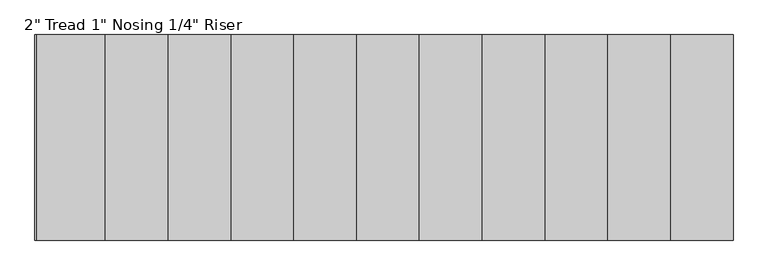
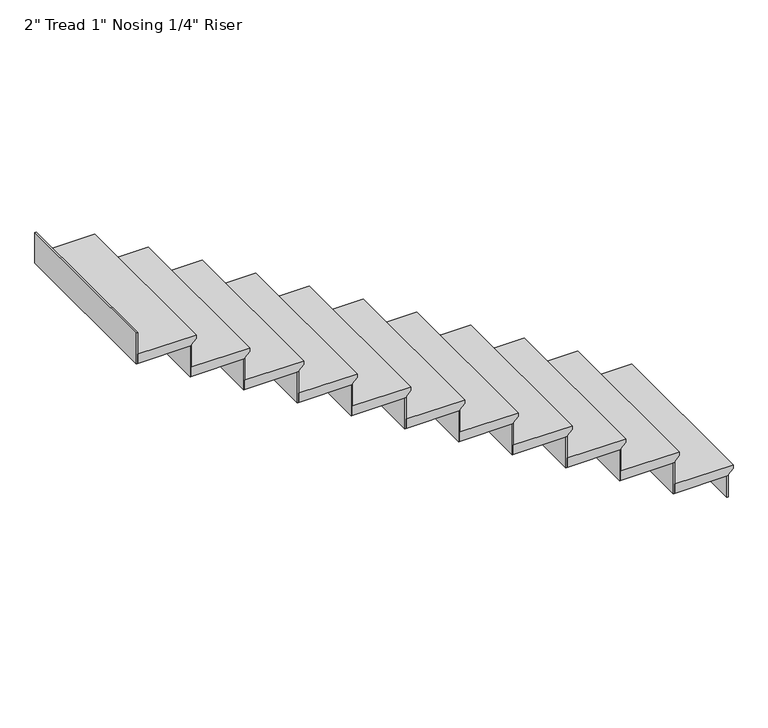
"""IFC4 building model written with IfcOpenShell, lengths in millimetres: stair flight geometry."""

from ifc_helpers import new_model, si_unit, frame, origin, origin_with_axes, place, context, project, spatial, polyline, outline, extrude, source, transform, mapped, element, save


def stair_flight_75b00a3b(model_context):
    return source(origin(), model_context, "Body", "SweptSolid", [
        extrude(outline(polyline([(169.3333333, -7020.8836698), (169.3333333, -7325.6836698), (118.5333333, -7325.6836698), (118.5333333, -7046.2836698), (124.8833333, -7046.2836698), (150.2833333, -7020.8836698), (169.3333333, -7020.8836698)])), frame((0.0, -870.1093225, 0.0), z_axis=(0.0, 1.0, 0.0), x_axis=(0.0, 0.0, 1.0)), (0.0, 0.0, 1.0), 914.4),
        extrude(outline(polyline([(-7052.6336698, 44.2906775), (-7046.2836698, 44.2906775), (-7046.2836698, -870.1093225), (-7052.6336698, -870.1093225), (-7052.6336698, 44.2906775)])), origin_with_axes(), (0.0, 0.0, 1.0), 118.5333333),
        extrude(outline(polyline([(-7332.0336698, 44.2906775), (-7325.6836698, 44.2906775), (-7325.6836698, -870.1093225), (-7332.0336698, -870.1093225), (-7332.0336698, 44.2906775)])), frame((0.0, 0.0, 118.5333333), z_axis=(0.0, 0.0, 1.0), x_axis=(1.0, 0.0, 0.0)), (0.0, 0.0, 1.0), 169.3333333),
        extrude(outline(polyline([(338.6666667, -7300.2836698), (338.6666667, -7605.0836698), (287.8666667, -7605.0836698), (287.8666667, -7325.6836698), (294.2166667, -7325.6836698), (319.6166667, -7300.2836698), (338.6666667, -7300.2836698)])), frame((0.0, -870.1093225, 0.0), z_axis=(0.0, 1.0, 0.0), x_axis=(0.0, 0.0, 1.0)), (0.0, 0.0, 1.0), 914.4),
        extrude(outline(polyline([(-7611.4336698, 44.2906775), (-7605.0836698, 44.2906775), (-7605.0836698, -870.1093225), (-7611.4336698, -870.1093225), (-7611.4336698, 44.2906775)])), frame((0.0, 0.0, 287.8666667), z_axis=(0.0, 0.0, 1.0), x_axis=(1.0, 0.0, 0.0)), (0.0, 0.0, 1.0), 169.3333333),
        extrude(outline(polyline([(508.0, -7579.6836698), (508.0, -7884.4836698), (457.2, -7884.4836698), (457.2, -7605.0836698), (463.55, -7605.0836698), (488.95, -7579.6836698), (508.0, -7579.6836698)])), frame((0.0, -870.1093225, 0.0), z_axis=(0.0, 1.0, 0.0), x_axis=(0.0, 0.0, 1.0)), (0.0, 0.0, 1.0), 914.4),
        extrude(outline(polyline([(-7890.8336698, 44.2906775), (-7884.4836698, 44.2906775), (-7884.4836698, -870.1093225), (-7890.8336698, -870.1093225), (-7890.8336698, 44.2906775)])), frame((0.0, 0.0, 457.2), z_axis=(0.0, 0.0, 1.0), x_axis=(1.0, 0.0, 0.0)), (0.0, 0.0, 1.0), 169.3333333),
        extrude(outline(polyline([(677.3333333, -7859.0836698), (677.3333333, -8163.8836698), (626.5333333, -8163.8836698), (626.5333333, -7884.4836698), (632.8833333, -7884.4836698), (658.2833333, -7859.0836698), (677.3333333, -7859.0836698)])), frame((0.0, -870.1093225, 0.0), z_axis=(0.0, 1.0, 0.0), x_axis=(0.0, 0.0, 1.0)), (0.0, 0.0, 1.0), 914.4),
        extrude(outline(polyline([(-8170.2336698, 44.2906775), (-8163.8836698, 44.2906775), (-8163.8836698, -870.1093225), (-8170.2336698, -870.1093225), (-8170.2336698, 44.2906775)])), frame((0.0, 0.0, 626.5333333), z_axis=(0.0, 0.0, 1.0), x_axis=(1.0, 0.0, 0.0)), (0.0, 0.0, 1.0), 169.3333333),
        extrude(outline(polyline([(846.6666667, -8138.4836698), (846.6666667, -8443.2836698), (795.8666667, -8443.2836698), (795.8666667, -8163.8836698), (802.2166667, -8163.8836698), (827.6166667, -8138.4836698), (846.6666667, -8138.4836698)])), frame((0.0, -870.1093225, 0.0), z_axis=(0.0, 1.0, 0.0), x_axis=(0.0, 0.0, 1.0)), (0.0, 0.0, 1.0), 914.4),
        extrude(outline(polyline([(-8449.6336698, 44.2906775), (-8443.2836698, 44.2906775), (-8443.2836698, -870.1093225), (-8449.6336698, -870.1093225), (-8449.6336698, 44.2906775)])), frame((0.0, 0.0, 795.8666667), z_axis=(0.0, 0.0, 1.0), x_axis=(1.0, 0.0, 0.0)), (0.0, 0.0, 1.0), 169.3333333),
        extrude(outline(polyline([(1016.0, -8417.8836698), (1016.0, -8722.6836698), (965.2, -8722.6836698), (965.2, -8443.2836698), (971.55, -8443.2836698), (996.95, -8417.8836698), (1016.0, -8417.8836698)])), frame((0.0, -870.1093225, 0.0), z_axis=(0.0, 1.0, 0.0), x_axis=(0.0, 0.0, 1.0)), (0.0, 0.0, 1.0), 914.4),
        extrude(outline(polyline([(-8729.0336698, 44.2906775), (-8722.6836698, 44.2906775), (-8722.6836698, -870.1093225), (-8729.0336698, -870.1093225), (-8729.0336698, 44.2906775)])), frame((0.0, 0.0, 965.2), z_axis=(0.0, 0.0, 1.0), x_axis=(1.0, 0.0, 0.0)), (0.0, 0.0, 1.0), 169.3333333),
        extrude(outline(polyline([(1185.3333333, -8697.2836698), (1185.3333333, -9002.0836698), (1134.5333333, -9002.0836698), (1134.5333333, -8722.6836698), (1140.8833333, -8722.6836698), (1166.2833333, -8697.2836698), (1185.3333333, -8697.2836698)])), frame((0.0, -870.1093225, 0.0), z_axis=(0.0, 1.0, 0.0), x_axis=(0.0, 0.0, 1.0)), (0.0, 0.0, 1.0), 914.4),
        extrude(outline(polyline([(-9008.4336698, 44.2906775), (-9002.0836698, 44.2906775), (-9002.0836698, -870.1093225), (-9008.4336698, -870.1093225), (-9008.4336698, 44.2906775)])), frame((0.0, 0.0, 1134.5333333), z_axis=(0.0, 0.0, 1.0), x_axis=(1.0, 0.0, 0.0)), (0.0, 0.0, 1.0), 169.3333333),
        extrude(outline(polyline([(1354.6666667, -8976.6836698), (1354.6666667, -9281.4836698), (1303.8666667, -9281.4836698), (1303.8666667, -9002.0836698), (1310.2166667, -9002.0836698), (1335.6166667, -8976.6836698), (1354.6666667, -8976.6836698)])), frame((0.0, -870.1093225, 0.0), z_axis=(0.0, 1.0, 0.0), x_axis=(0.0, 0.0, 1.0)), (0.0, 0.0, 1.0), 914.4),
        extrude(outline(polyline([(-9287.8336698, 44.2906775), (-9281.4836698, 44.2906775), (-9281.4836698, -870.1093225), (-9287.8336698, -870.1093225), (-9287.8336698, 44.2906775)])), frame((0.0, 0.0, 1303.8666667), z_axis=(0.0, 0.0, 1.0), x_axis=(1.0, 0.0, 0.0)), (0.0, 0.0, 1.0), 169.3333333),
        extrude(outline(polyline([(1524.0, -9256.0836698), (1524.0, -9560.8836698), (1473.2, -9560.8836698), (1473.2, -9281.4836698), (1479.55, -9281.4836698), (1504.95, -9256.0836698), (1524.0, -9256.0836698)])), frame((0.0, -870.1093225, 0.0), z_axis=(0.0, 1.0, 0.0), x_axis=(0.0, 0.0, 1.0)), (0.0, 0.0, 1.0), 914.4),
        extrude(outline(polyline([(-9567.2336698, 44.2906775), (-9560.8836698, 44.2906775), (-9560.8836698, -870.1093225), (-9567.2336698, -870.1093225), (-9567.2336698, 44.2906775)])), frame((0.0, 0.0, 1473.2), z_axis=(0.0, 0.0, 1.0), x_axis=(1.0, 0.0, 0.0)), (0.0, 0.0, 1.0), 169.3333333),
        extrude(outline(polyline([(1693.3333333, -9535.4836698), (1693.3333333, -9840.2836698), (1642.5333333, -9840.2836698), (1642.5333333, -9560.8836698), (1648.8833333, -9560.8836698), (1674.2833333, -9535.4836698), (1693.3333333, -9535.4836698)])), frame((0.0, -870.1093225, 0.0), z_axis=(0.0, 1.0, 0.0), x_axis=(0.0, 0.0, 1.0)), (0.0, 0.0, 1.0), 914.4),
        extrude(outline(polyline([(-9846.6336698, 44.2906775), (-9840.2836698, 44.2906775), (-9840.2836698, -870.1093225), (-9846.6336698, -870.1093225), (-9846.6336698, 44.2906775)])), frame((0.0, 0.0, 1642.5333333), z_axis=(0.0, 0.0, 1.0), x_axis=(1.0, 0.0, 0.0)), (0.0, 0.0, 1.0), 169.3333333),
        extrude(outline(polyline([(-10126.0336698, 44.2906775), (-10119.6836698, 44.2906775), (-10119.6836698, -870.1093225), (-10126.0336698, -870.1093225), (-10126.0336698, 44.2906775)])), frame((0.0, 0.0, 1811.8666667), z_axis=(0.0, 0.0, 1.0), x_axis=(1.0, 0.0, 0.0)), (0.0, 0.0, 1.0), 169.3333333),
        extrude(outline(polyline([(1862.6666667, -9814.8836698), (1862.6666667, -10119.6836698), (1811.8666667, -10119.6836698), (1811.8666667, -9840.2836698), (1818.2166667, -9840.2836698), (1843.6166667, -9814.8836698), (1862.6666667, -9814.8836698)])), frame((0.0, -870.1093225, 0.0), z_axis=(0.0, 1.0, 0.0), x_axis=(0.0, 0.0, 1.0)), (0.0, 0.0, 1.0), 914.4),
    ])


if __name__ == "__main__":
    model = new_model("IFC4")
    model_context = context("Model", 3, world=origin())
    ifc_project = project(units=[si_unit("LENGTHUNIT", "METRE", prefix="MILLI")], contexts=[model_context])
    site = spatial("IfcSite", under=ifc_project)
    building = spatial("IfcBuilding", under=site)
    placement = place(None, origin())
    stair_flight_shape = stair_flight_75b00a3b(model_context)
    element("IfcStairFlight", 1, ObjectType="2\" Tread 1\" Nosing 1/4\" Riser", at=placement, inside=building, context=model_context, shape_type="MappedRepresentation", body=[
        mapped(stair_flight_shape, transform((0.0, 0.0, 0.0), x_axis=(1.0, 0.0, 0.0), y_axis=(0.0, 1.0, 0.0), z_axis=(0.0, 0.0, 1.0))),
    ])
    save(model, "model.ifc")
